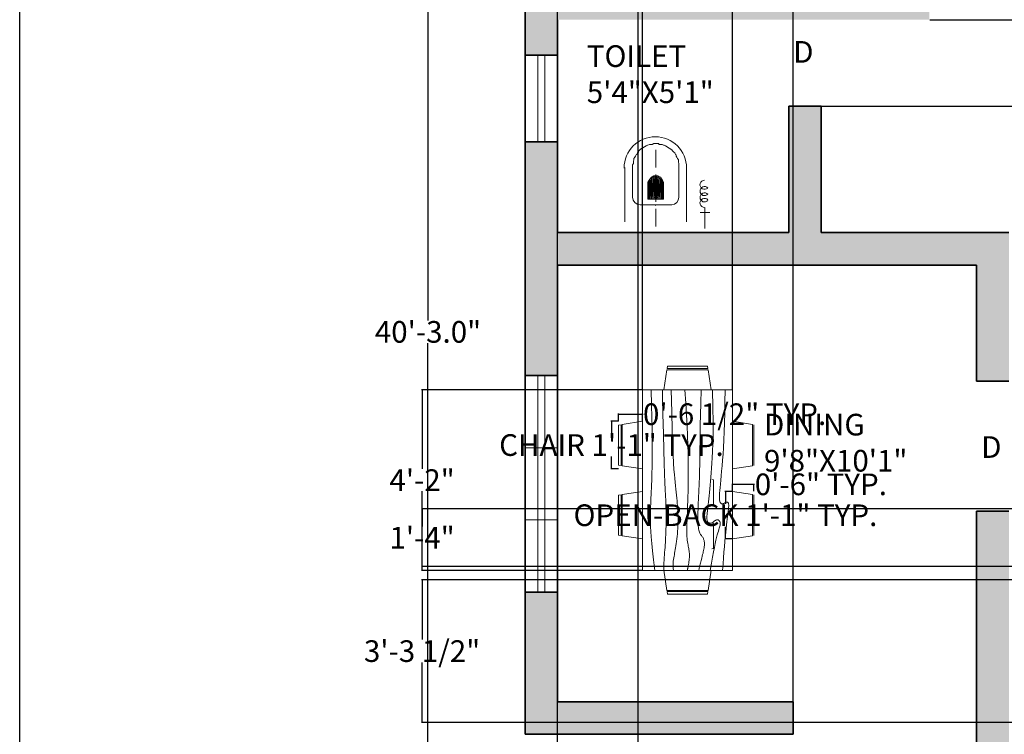
# Model space of a CAD drawing. Units: inches. Extents: x 2552 to 3196, y 4736 to 5443.
# Tile 2 of 8: x 2552 to 2824, y 4938 to 5136. Entities that reach past the tile are written whole.
import ezdxf

# ---------------------------------------------------------------- set-up
doc = ezdxf.new("R2010")
doc.units = ezdxf.units.IN
doc.header["$MEASUREMENT"] = 0
for name, color, linetype, lineweight in [('A-ANNO-DIMS', 2, 'Continuous', 18), ('A-ANNO-TTLB', 7, 'Continuous', 25), ('A-AREA-IDEN', 7, 'Continuous', 18), ('A-DOOR-IDEN', 7, 'Continuous', 18), ('A-FLOR-FIXT', 7, 'Continuous', 18), ('A-FURN', 8, 'Continuous', 18), ('A-GLAZ', 4, 'Continuous', 18), ('A-WALL', 7, 'Continuous', 35)]:
    doc.layers.add(name, color=color, linetype=linetype, lineweight=lineweight)
doc.layers.add('A-WALL-PATT', color=30, linetype='Continuous', lineweight=13, true_color=0xf8991e)
doc.styles.get("Standard").update_dxf_attribs({"font": 'arial.ttf'})
doc.dimstyles.get("Standard").update_dxf_attribs({"dimtxt": 6, "dimasz": 0.18, "dimexe": 0.18, "dimexo": 0.0625, "dimgap": 0.09, "dimtad": 0, "dimtih": 1, "dimtoh": 1, "dimdec": 1, "dimzin": 0, "dimdsep": 46, "dimlunit": 3, "dimtxsty": 'Standard', "dimcen": 0.09, "dimadec": 0, "dimazin": 0, "dimtfac": 1, "dimtdec": 1, "dimtofl": 0, "dimtmove": 0, "dimatfit": 3, "dimfxl": 1, "dimtolj": 1, "dimtzin": 0, "dimarcsym": 0})

# ---------------------------------------------------------------- blocks, each defined once
blk = doc.blocks.new('*D1')
at = {"layer": 'A-ANNO-DIMS', "color": 0, "lineweight": -2, "transparency": 16777216}
for p, q in [((2691.59, 5291.32), (2664.57, 5291.32)), ((2664.75, 5291.14), (2664.75, 5052.97)), ((2664.75, 4808.5), (2664.75, 5046.66)), ((2691.59, 4808.32), (2664.57, 4808.32))]:
    blk.add_line(p, q, dxfattribs=at)
at = {"layer": 'A-ANNO-DIMS', "color": 0, "transparency": 16777216}
for points in [[(2664.72, 5291.14), (2664.78, 5291.14), (2664.75, 5291.32)], [(2664.72, 4808.5), (2664.78, 4808.5), (2664.75, 4808.32)]]:
    blk.add_solid(points, dxfattribs=at)
at = {"layer": 'Defpoints', "color": 0, "transparency": 16777216}
for p in [(2691.66, 5291.32), (2664.75, 4808.32), (2691.66, 4808.32)]:
    blk.add_point(p, dxfattribs=at)
at = {"layer": 'A-ANNO-DIMS', "color": 0, "transparency": 16777216, "insert": (2664.75, 5049.82), "char_height": 6, "attachment_point": 5}
blk.add_mtext('\\A1;40\'-3.0"', dxfattribs=at)
blk = doc.blocks.new('WIN-60IN-THREE-LIGHT')
for p, q in [((60, 9), (0, 9)), ((20, 9), (20, 0)), ((40, 0), (40, 9)), ((60, 5.5), (0, 5.5)), ((0, 3.5), (60, 3.5)), ((0, 0), (60, 0))]:
    blk.add_line(p, q)
blk = doc.blocks.new('VENT-24IN')
for p, q in [((24, 9), (0, 9)), ((24, 5.5), (0, 5.5)), ((0, 3.5), (24, 3.5)), ((0, 0), (24, 0))]:
    blk.add_line(p, q)
blk = doc.blocks.new('WC-SQUAT')
h = blk.add_hatch(color=256)
h.paths.add_polyline_path([(7.21, 8.12), (7.21, 13.81), (7.05, 8.12)])
h.paths.add_polyline_path([(7.21, 13.81), (7.05, 8.12), (7.05, 13.58)])
h = blk.add_hatch(color=256)
h.paths.add_polyline_path([(7.59, 8.12), (7.59, 14.19), (7.21, 8.12)])
h.paths.add_polyline_path([(7.59, 14.19), (7.21, 8.12), (7.21, 13.81)])
h = blk.add_hatch(color=256)
h.paths.add_polyline_path([(7.81, 8.12), (7.81, 14.34), (7.59, 8.12)])
h.paths.add_polyline_path([(7.81, 14.34), (7.59, 8.12), (7.59, 14.19)])
h = blk.add_hatch(color=256)
h.paths.add_polyline_path([(8.19, 8.12), (8.19, 14.56), (7.81, 8.12)])
h.paths.add_polyline_path([(8.19, 14.56), (7.81, 8.12), (7.81, 14.34)])
h = blk.add_hatch(color=256)
h.paths.add_polyline_path([(8.57, 8.12), (8.57, 14.56), (8.19, 8.12)])
h.paths.add_polyline_path([(8.57, 14.56), (8.19, 8.12), (8.19, 14.56)])
h = blk.add_hatch(color=256)
h.paths.add_polyline_path([(8.95, 8.12), (8.95, 14.56), (8.57, 8.12)])
h.paths.add_polyline_path([(8.95, 14.56), (8.57, 8.12), (8.57, 14.56)])
h = blk.add_hatch(color=256)
h.paths.add_polyline_path([(9.33, 8.12), (9.33, 14.56), (8.95, 8.12)])
h.paths.add_polyline_path([(9.33, 14.56), (8.95, 8.12), (8.95, 14.56)])
h = blk.add_hatch(color=256)
h.paths.add_polyline_path([(9.71, 8.12), (9.71, 14.34), (9.33, 8.12)])
h.paths.add_polyline_path([(9.71, 14.34), (9.33, 8.12), (9.33, 14.56)])
h = blk.add_hatch(color=256)
h.paths.add_polyline_path([(10.16, 8.12), (10.16, 14.19), (9.71, 8.12)])
h.paths.add_polyline_path([(10.16, 14.19), (9.71, 8.12), (9.71, 14.34)])
h = blk.add_hatch(color=256)
h.paths.add_polyline_path([(10.32, 8.12), (10.32, 13.81), (10.16, 8.12)])
h.paths.add_polyline_path([(10.32, 13.81), (10.16, 8.12), (10.16, 14.19)])
h = blk.add_hatch(color=256)
h.paths.add_polyline_path([(10.54, 8.12), (10.54, 13.58), (10.32, 8.12)])
h.paths.add_polyline_path([(10.54, 13.58), (10.32, 8.12), (10.32, 13.81)])
h = blk.add_hatch(color=256)
h.paths.add_polyline_path([(6.83, 8.12), (6.83, 13.2), (6.6, 8.12)])
h.paths.add_polyline_path([(6.83, 13.2), (6.6, 8.12), (6.6, 12.82)])
h.paths.add_polyline_path([(6.6, 8.12), (6.6, 12.82), (6.6, 12.44)])
h = blk.add_hatch(color=256)
h.paths.add_polyline_path([(7.05, 8.12), (7.05, 13.58), (6.83, 8.12)])
h.paths.add_polyline_path([(7.05, 13.58), (6.83, 8.12), (6.83, 13.2)])
h = blk.add_hatch(color=256)
h.paths.add_polyline_path([(10.7, 8.12), (10.7, 13.2), (10.54, 8.12)])
h.paths.add_polyline_path([(10.7, 13.2), (10.54, 8.12), (10.54, 13.58)])
h = blk.add_hatch(color=256)
h.paths.add_polyline_path([(10.92, 8.12), (10.92, 12.82), (10.7, 8.12)])
h.paths.add_polyline_path([(10.92, 12.82), (10.7, 8.12), (10.7, 13.2)])
for points in [[(2.35, 15.93), (2.35, 16.69), (2.35, 17.3), (2.35, 17.67), (2.58, 18.05), (2.58, 18.43), (2.58, 18.66), (2.73, 19.04), (2.73, 19.42), (2.96, 19.8), (3.11, 20.03), (3.34, 20.41), (3.49, 20.56), (3.72, 20.94), (3.94, 21.16), (4.1, 21.54), (4.32, 21.77), (4.48, 21.92), (4.85, 22.15), (5.08, 22.3), (5.46, 22.53), (5.69, 22.68), (6.07, 22.91), (6.45, 23.14), (6.6, 23.14), (7.05, 23.29), (7.43, 23.29), (7.81, 23.29), (8.19, 23.52), (8.8, 23.52), (9.56, 23.52), (9.71, 23.29), (10.16, 23.29), (10.54, 23.29), (10.92, 23.14), (11.08, 23.14), (11.45, 22.91), (11.91, 22.68), (12.06, 22.53), (12.44, 22.3), (12.67, 22.15), (13.05, 21.92), (13.2, 21.77), (13.43, 21.54), (13.81, 21.16), (14.03, 20.94), (14.19, 20.56), (14.41, 20.41), (14.41, 20.03), (14.56, 19.8), (14.79, 19.42), (15.02, 19.04), (15.02, 18.66), (15.02, 18.43), (15.17, 18.05), (15.17, 17.67), (15.17, 17.3), (15.17, 16.69), (15.17, 15.93)], [(8.8, 16.92), (8.8, 21.77), (8.8, 21.77)], [(0.23, 1.9), (0.23, 16.92), (0.23, 16.92)], [(17.3, 1.9), (17.3, 16.92), (17.3, 16.92)], [(2.35, 8.72), (2.35, 15.93), (2.35, 15.93)], [(8.8, 7.36), (8.8, 14.94), (8.8, 14.94)], [(15.17, 8.72), (15.17, 15.93), (15.17, 15.93)], [(6.6, 8.12), (6.6, 12.44), (6.6, 12.44)], [(10.92, 8.12), (10.92, 12.44), (10.92, 12.44)], [(8.34, 8.57), (8.57, 8.57), (8.8, 8.57)], [(8.34, 8.57), (8.34, 8.5), (8.34, 8.5)], [(8.8, 8.57), (8.72, 8.5), (8.72, 8.5)], [(8.8, 8.57), (8.95, 8.57), (9.18, 8.57)], [(9.18, 8.57), (9.18, 8.5), (9.18, 8.5)], [(4.48, 6.6), (13.2, 6.6), (13.2, 6.6)], [(6.6, 8.12), (10.92, 8.12), (10.92, 8.12)], [(8.8, 6.37), (8.72, 6.37), (8.72, 6.37)], [(8.8, 0.61), (8.8, 5.46), (8.8, 5.46)], [(22.4, 0), (22.4, 5.84), (22.4, 5.84)], [(21.04, 4.48), (23.77, 4.48), (23.77, 4.48)]]:
    blk.add_lwpolyline(points)
for points in [[(7.21, 8.12), (7.21, 13.81), (7.05, 8.12)], [(7.21, 13.81), (7.05, 8.12), (7.05, 13.58)], [(7.59, 8.12), (7.59, 14.19), (7.21, 8.12)], [(7.59, 14.19), (7.21, 8.12), (7.21, 13.81)], [(7.81, 8.12), (7.81, 14.34), (7.59, 8.12)], [(7.81, 14.34), (7.59, 8.12), (7.59, 14.19)], [(8.19, 8.12), (8.19, 14.56), (7.81, 8.12)], [(8.19, 14.56), (7.81, 8.12), (7.81, 14.34)], [(8.57, 8.12), (8.57, 14.56), (8.19, 8.12)], [(8.57, 14.56), (8.19, 8.12), (8.19, 14.56)], [(8.95, 8.12), (8.95, 14.56), (8.57, 8.12)], [(8.95, 14.56), (8.57, 8.12), (8.57, 14.56)], [(9.33, 8.12), (9.33, 14.56), (8.95, 8.12)], [(9.33, 14.56), (8.95, 8.12), (8.95, 14.56)], [(9.71, 14.34), (9.33, 8.12), (9.33, 14.56)], [(9.71, 8.12), (9.71, 14.34), (9.33, 8.12)], [(10.16, 14.19), (9.71, 8.12), (9.71, 14.34)], [(10.16, 8.12), (10.16, 14.19), (9.71, 8.12)], [(10.32, 13.81), (10.16, 8.12), (10.16, 14.19)], [(10.32, 8.12), (10.32, 13.81), (10.16, 8.12)], [(10.54, 13.58), (10.32, 8.12), (10.32, 13.81)], [(6.83, 8.12), (6.83, 13.2), (6.6, 8.12)], [(6.83, 13.2), (6.6, 8.12), (6.6, 12.82)], [(6.6, 8.12), (6.6, 12.82), (6.6, 12.44)], [(6.6, 12.82), (6.6, 8.12), (6.6, 8.12)], [(7.05, 8.12), (7.05, 13.58), (6.83, 8.12)], [(7.05, 13.58), (6.83, 8.12), (6.83, 13.2)], [(10.54, 8.12), (10.54, 13.58), (10.32, 8.12)], [(10.7, 13.2), (10.54, 8.12), (10.54, 13.58)], [(10.7, 8.12), (10.7, 13.2), (10.54, 8.12)], [(10.92, 12.82), (10.7, 8.12), (10.7, 13.2)], [(10.92, 8.12), (10.92, 12.82), (10.7, 8.12)], [(10.92, 12.44), (10.92, 8.12), (10.92, 12.82)], [(10.92, 8.12), (10.92, 12.44)]]:
    blk.add_lwpolyline(points, close=True)
for points, knots in [([(17.3, 16.76), (17.3, 21.54), (13.43, 25.41), (8.65, 25.41), (8.65, 25.41), (3.87, 25.41), (0, 21.54), (0, 16.76)], [0, 0, 0, 0, 0.125, 0.125, 0.125, 0.125001, 1, 1, 1, 1]), ([(10.7, 12.29), (10.7, 13.43), (9.79, 14.34), (8.65, 14.34), (8.65, 14.34), (7.51, 14.34), (6.6, 13.43), (6.6, 12.29)], [0, 0, 0, 0, 0.125, 0.125, 0.125, 0.125001, 1, 1, 1, 1]), ([(22.25, 13.43), (21.72, 13.43), (21.19, 12.97), (21.04, 12.44), (21.04, 12.44), (20.88, 11.91), (21.19, 11.3), (21.64, 11), (21.64, 11), (22.17, 10.77), (22.78, 10.85), (23.16, 11.23)], [0, 0, 0, 0, 0.083333, 0.083333, 0.083333, 0.083334, 0.166667, 0.166667, 0.166667, 0.166668, 1, 1, 1, 1]), ([(23.23, 11.23), (22.86, 11.61), (22.32, 11.76), (21.79, 11.53), (21.79, 11.53), (21.34, 11.38), (21.04, 10.92), (21.04, 10.39), (21.04, 10.39), (21.04, 9.86), (21.34, 9.41), (21.79, 9.18), (21.79, 9.18), (22.32, 9.03), (22.86, 9.18), (23.23, 9.56)], [0, 0, 0, 0, 0.0625, 0.0625, 0.0625, 0.062501, 0.125, 0.125, 0.125, 0.125001, 0.1875, 0.1875, 0.1875, 0.187501, 1, 1, 1, 1]), ([(23.23, 7.96), (22.86, 8.34), (22.17, 8.5), (21.72, 8.19), (21.72, 8.19), (21.19, 7.89), (20.88, 7.36), (21.04, 6.75), (21.04, 6.75), (21.19, 6.22), (21.72, 5.84), (22.25, 5.84)], [0, 0, 0, 0, 0.083333, 0.083333, 0.083333, 0.083334, 0.166667, 0.166667, 0.166667, 0.166668, 1, 1, 1, 1]), ([(23.16, 9.48), (22.86, 9.86), (22.25, 10.01), (21.79, 9.79), (21.79, 9.79), (21.34, 9.63), (21.04, 9.1), (21.04, 8.65), (21.04, 8.65), (21.04, 8.12), (21.34, 7.66), (21.79, 7.43), (21.79, 7.43), (22.32, 7.28), (22.86, 7.43), (23.23, 7.81)], [0, 0, 0, 0, 0.0625, 0.0625, 0.0625, 0.062501, 0.125, 0.125, 0.125, 0.125001, 0.1875, 0.1875, 0.1875, 0.187501, 1, 1, 1, 1])]:
    blk.add_open_spline(points, degree=3, knots=knots)
for points in [[(2.35, 8.65), (2.35, 7.51), (3.26, 6.6), (4.4, 6.6)], [(13.12, 6.6), (14.26, 6.6), (15.17, 7.51), (15.17, 8.65)]]:
    blk.add_open_spline(points, degree=3)
blk = doc.blocks.new('CHAIR-DINING')
for p, q in [((0, 12.14), (0.69, 12.24)), ((0, 12.14), (0, 1.03)), ((0.69, 0.92), (0.69, 12.24)), ((1.04, 12.3), (6.6, 13.17)), ((1.04, 12.3), (1.04, 0.86)), ((0.69, 0.92), (0, 1.03)), ((6.6, 0), (1.04, 0.87))]:
    blk.add_line(p, q)
blk = doc.blocks.new('CHAIR-DINING-OPEN-BACK')
for p, q in [((5.55, 12.3), (0, 13.17)), ((5.55, 12.3), (5.55, 0.86)), ((5.9, 0.92), (5.9, 12.24)), ((0, 0), (5.55, 0.87))]:
    blk.add_line(p, q)
blk = doc.blocks.new('*D17')
at = {"layer": 'A-ANNO-DIMS', "color": 0, "lineweight": -2, "transparency": 16777216}
for p, q in [((2717.48, 5025.04), (2715.39, 5025.04)), ((2715.57, 5024.86), (2715.57, 5021.65)), ((2715.57, 5012.05), (2715.57, 5015.26)), ((2717.48, 5011.87), (2715.39, 5011.87))]:
    blk.add_line(p, q, dxfattribs=at)
at = {"layer": 'A-ANNO-DIMS', "color": 0, "transparency": 16777216}
for points in [[(2715.54, 5024.86), (2715.6, 5024.86), (2715.57, 5025.04)], [(2715.54, 5012.05), (2715.6, 5012.05), (2715.57, 5011.87)]]:
    blk.add_solid(points, dxfattribs=at)
at = {"layer": 'Defpoints', "color": 0, "transparency": 16777216}
for p in [(2715.57, 5025.04), (2717.54, 5025.04), (2717.54, 5011.87)]:
    blk.add_point(p, dxfattribs=at)
at = {"layer": 'A-ANNO-DIMS', "color": 0, "transparency": 16777216, "insert": (2715.57, 5018.46), "char_height": 6, "attachment_point": 5}
blk.add_mtext('\\A1;CHAIR 1\'-1" TYP.', dxfattribs=at)
blk = doc.blocks.new('*D18')
at = {"layer": 'A-ANNO-DIMS', "color": 0, "lineweight": -2, "transparency": 16777216}
for p, q in [((2717.54, 5025.1), (2717.54, 5027.19)), ((2717.72, 5027.01), (2723.96, 5027.01)), ((2724.14, 5025.1), (2724.14, 5027.19)), ((2724.14, 5027.01), (2724.32, 5027.01))]:
    blk.add_line(p, q, dxfattribs=at)
at = {"layer": 'A-ANNO-DIMS', "color": 0, "transparency": 16777216}
for points in [[(2717.72, 5027.04), (2717.72, 5026.98), (2717.54, 5027.01)], [(2723.96, 5027.04), (2723.96, 5026.98), (2724.14, 5027.01)]]:
    blk.add_solid(points, dxfattribs=at)
at = {"layer": 'Defpoints', "color": 0, "transparency": 16777216}
for p in [(2724.14, 5027.01), (2717.54, 5025.04), (2724.14, 5025.04)]:
    blk.add_point(p, dxfattribs=at)
at = {"layer": 'A-ANNO-DIMS', "color": 0, "transparency": 16777216, "insert": (2749.68, 5027.01), "char_height": 6, "attachment_point": 5}
blk.add_mtext('\\A1;0\'-6 1/2" TYP.', dxfattribs=at)
blk = doc.blocks.new('*D19')
at = {"layer": 'A-ANNO-DIMS', "color": 0, "lineweight": -2, "transparency": 16777216}
for p, q in [((2749.06, 5005.61), (2746.97, 5005.61)), ((2747.15, 5005.43), (2747.15, 5002.22)), ((2747.15, 4992.62), (2747.15, 4995.83)), ((2749.06, 4992.44), (2746.97, 4992.44))]:
    blk.add_line(p, q, dxfattribs=at)
at = {"layer": 'A-ANNO-DIMS', "color": 0, "transparency": 16777216}
for points in [[(2747.12, 5005.43), (2747.18, 5005.43), (2747.15, 5005.61)], [(2747.12, 4992.62), (2747.18, 4992.62), (2747.15, 4992.44)]]:
    blk.add_solid(points, dxfattribs=at)
at = {"layer": 'Defpoints', "color": 0, "transparency": 16777216}
for p in [(2747.15, 5005.61), (2749.12, 5005.61), (2749.12, 4992.44)]:
    blk.add_point(p, dxfattribs=at)
at = {"layer": 'A-ANNO-DIMS', "color": 0, "transparency": 16777216, "insert": (2747.15, 4999.02), "char_height": 6, "attachment_point": 5}
blk.add_mtext('\\A1;OPEN-BACK 1\'-1" TYP.', dxfattribs=at)
blk = doc.blocks.new('*D20')
at = {"layer": 'A-ANNO-DIMS', "color": 0, "lineweight": -2, "transparency": 16777216}
for p, q in [((2749.12, 5005.67), (2749.12, 5007.76)), ((2749.3, 5007.58), (2754.84, 5007.58)), ((2755.02, 5005.67), (2755.02, 5007.76)), ((2755.02, 5007.58), (2755.2, 5007.58))]:
    blk.add_line(p, q, dxfattribs=at)
at = {"layer": 'A-ANNO-DIMS', "color": 0, "transparency": 16777216}
for points in [[(2749.3, 5007.61), (2749.3, 5007.55), (2749.12, 5007.58)], [(2754.84, 5007.61), (2754.84, 5007.55), (2755.02, 5007.58)]]:
    blk.add_solid(points, dxfattribs=at)
at = {"layer": 'Defpoints', "color": 0, "transparency": 16777216}
for p in [(2755.02, 5007.58), (2749.12, 5005.61), (2755.02, 5005.61)]:
    blk.add_point(p, dxfattribs=at)
at = {"layer": 'A-ANNO-DIMS', "color": 0, "transparency": 16777216, "insert": (2773.58, 5007.58), "char_height": 6, "attachment_point": 5}
blk.add_mtext('\\A1;0\'-6" TYP.', dxfattribs=at)
blk = doc.blocks.new('*D26')
at = {"layer": 'A-ANNO-DIMS', "color": 0, "lineweight": -2, "transparency": 16777216}
for p, q in [((2803.72, 5136.32), (3083.39, 5136.32)), ((3083.21, 5136.14), (3083.21, 5127.47)), ((3083.21, 5112.5), (3083.21, 5121.16)), ((2773.72, 5112.32), (3083.39, 5112.32))]:
    blk.add_line(p, q, dxfattribs=at)
at = {"layer": 'A-ANNO-DIMS', "color": 0, "transparency": 16777216}
for points in [[(3083.18, 5136.14), (3083.24, 5136.14), (3083.21, 5136.32)], [(3083.18, 5112.5), (3083.24, 5112.5), (3083.21, 5112.32)]]:
    blk.add_solid(points, dxfattribs=at)
at = {"layer": 'Defpoints', "color": 0, "transparency": 16777216}
for p in [(2803.66, 5136.32), (2773.66, 5112.32), (3083.21, 5112.32)]:
    blk.add_point(p, dxfattribs=at)
at = {"layer": 'A-ANNO-DIMS', "color": 0, "transparency": 16777216, "insert": (3083.21, 5124.32), "char_height": 6, "attachment_point": 5}
blk.add_mtext('\\A1;2\'-0"', dxfattribs=at)
blk = doc.blocks.new('*D29')
at = {"layer": 'A-ANNO-DIMS', "color": 0, "lineweight": -2, "transparency": 16777216}
for p, q in [((2724.14, 5033.79), (2724.14, 5320.05)), ((2724.32, 5319.87), (2728.51, 5319.87)), ((2748.94, 5319.87), (2744.75, 5319.87)), ((2749.12, 5033.79), (2749.12, 5320.05))]:
    blk.add_line(p, q, dxfattribs=at)
at = {"layer": 'A-ANNO-DIMS', "color": 0, "transparency": 16777216}
for points in [[(2724.32, 5319.9), (2724.32, 5319.84), (2724.14, 5319.87)], [(2748.94, 5319.9), (2748.94, 5319.84), (2749.12, 5319.87)]]:
    blk.add_solid(points, dxfattribs=at)
at = {"layer": 'Defpoints', "color": 0, "transparency": 16777216}
for p in [(2749.12, 5319.87), (2724.14, 5033.73), (2749.12, 5033.73)]:
    blk.add_point(p, dxfattribs=at)
at = {"layer": 'A-ANNO-DIMS', "color": 0, "transparency": 16777216, "insert": (2736.63, 5319.87), "char_height": 6, "attachment_point": 5}
blk.add_mtext('\\A1;2\'-1"', dxfattribs=at)
blk = doc.blocks.new('*D30')
at = {"layer": 'A-ANNO-DIMS', "color": 0, "lineweight": -2, "transparency": 16777216}
for p, q in [((2724.07, 5033.73), (2662.93, 5033.73)), ((2663.11, 5033.55), (2663.11, 5011.84)), ((2663.11, 4983.93), (2663.11, 5005.64)), ((2724.07, 4983.75), (2662.93, 4983.75))]:
    blk.add_line(p, q, dxfattribs=at)
at = {"layer": 'A-ANNO-DIMS', "color": 0, "transparency": 16777216}
for points in [[(2663.08, 5033.55), (2663.14, 5033.55), (2663.11, 5033.73)], [(2663.08, 4983.93), (2663.14, 4983.93), (2663.11, 4983.75)]]:
    blk.add_solid(points, dxfattribs=at)
at = {"layer": 'Defpoints', "color": 0, "transparency": 16777216}
for p in [(2724.14, 5033.73), (2663.11, 4983.75), (2724.14, 4983.75)]:
    blk.add_point(p, dxfattribs=at)
at = {"layer": 'A-ANNO-DIMS', "color": 0, "transparency": 16777216, "insert": (2663.11, 5008.74), "char_height": 6, "attachment_point": 5}
blk.add_mtext('\\A1;4\'-2"', dxfattribs=at)
blk = doc.blocks.new('*D34')
at = {"layer": 'A-ANNO-DIMS', "color": 0, "lineweight": -2, "transparency": 16777216}
for p, q in [((2989.13, 5000.78), (2662.93, 5000.78)), ((2663.11, 5000.6), (2663.11, 4995.9)), ((2663.11, 4984.99), (2663.11, 4989.7)), ((2987.72, 4984.81), (2662.93, 4984.81))]:
    blk.add_line(p, q, dxfattribs=at)
at = {"layer": 'A-ANNO-DIMS', "color": 0, "transparency": 16777216}
for points in [[(2663.08, 5000.6), (2663.14, 5000.6), (2663.11, 5000.78)], [(2663.08, 4984.99), (2663.14, 4984.99), (2663.11, 4984.81)]]:
    blk.add_solid(points, dxfattribs=at)
at = {"layer": 'Defpoints', "color": 0, "transparency": 16777216}
for p in [(2663.11, 5000.78), (2989.19, 5000.78), (2987.78, 4984.81)]:
    blk.add_point(p, dxfattribs=at)
at = {"layer": 'A-ANNO-DIMS', "color": 0, "transparency": 16777216, "insert": (2663.11, 4992.8), "char_height": 6, "attachment_point": 5}
blk.add_mtext('\\A1;1\'-4"', dxfattribs=at)
blk = doc.blocks.new('*D35')
at = {"layer": 'A-ANNO-DIMS', "color": 0, "lineweight": -2, "transparency": 16777216}
for p, q in [((3026.66, 4981.14), (2662.93, 4981.14)), ((2663.11, 4980.96), (2663.11, 4964.56)), ((2663.11, 4941.78), (2663.11, 4958.17)), ((3026.66, 4941.6), (2662.93, 4941.6))]:
    blk.add_line(p, q, dxfattribs=at)
at = {"layer": 'A-ANNO-DIMS', "color": 0, "transparency": 16777216}
for points in [[(2663.08, 4980.96), (2663.14, 4980.96), (2663.11, 4981.14)], [(2663.08, 4941.78), (2663.14, 4941.78), (2663.11, 4941.6)]]:
    blk.add_solid(points, dxfattribs=at)
at = {"layer": 'Defpoints', "color": 0, "transparency": 16777216}
for p in [(3026.72, 4981.14), (2663.11, 4941.6), (3026.72, 4941.6)]:
    blk.add_point(p, dxfattribs=at)
at = {"layer": 'A-ANNO-DIMS', "color": 0, "transparency": 16777216, "insert": (2663.11, 4961.37), "char_height": 6, "attachment_point": 5}
blk.add_mtext('\\A1;3\'-3 1/2"', dxfattribs=at)
blk = doc.blocks.new('*D37')
at = {"layer": 'A-ANNO-DIMS', "color": 0, "lineweight": -2, "transparency": 16777216}
for p, q in [((2700.66, 4902.38), (2700.66, 5320.05)), ((2700.84, 5319.87), (2722.83, 5319.87)), ((2723.01, 4902.38), (2723.01, 5320.05)), ((2723.01, 5319.87), (2723.19, 5319.87))]:
    blk.add_line(p, q, dxfattribs=at)
at = {"layer": 'A-ANNO-DIMS', "color": 0, "transparency": 16777216}
for points in [[(2700.84, 5319.9), (2700.84, 5319.84), (2700.66, 5319.87)], [(2722.83, 5319.9), (2722.83, 5319.84), (2723.01, 5319.87)]]:
    blk.add_solid(points, dxfattribs=at)
at = {"layer": 'Defpoints', "color": 0, "transparency": 16777216}
for p in [(2723.01, 5319.87), (2700.66, 4902.32), (2723.01, 4902.32)]:
    blk.add_point(p, dxfattribs=at)
at = {"layer": 'A-ANNO-DIMS', "color": 0, "transparency": 16777216, "insert": (2740.29, 5319.87), "char_height": 6, "attachment_point": 5}
blk.add_mtext('\\A1;1\'-10 1/2"', dxfattribs=at)
blk = doc.blocks.new('*D40')
at = {"layer": 'A-ANNO-DIMS', "color": 0, "lineweight": -2, "transparency": 16777216}
for p, q in [((2700.66, 4947.38), (2700.66, 5320.05)), ((2700.84, 5319.87), (2718.23, 5319.87)), ((2765.73, 5319.87), (2748.34, 5319.87)), ((2765.91, 4947.38), (2765.91, 5320.05))]:
    blk.add_line(p, q, dxfattribs=at)
at = {"layer": 'A-ANNO-DIMS', "color": 0, "transparency": 16777216}
for points in [[(2700.84, 5319.9), (2700.84, 5319.84), (2700.66, 5319.87)], [(2765.73, 5319.9), (2765.73, 5319.84), (2765.91, 5319.87)]]:
    blk.add_solid(points, dxfattribs=at)
at = {"layer": 'Defpoints', "color": 0, "transparency": 16777216}
for p in [(2765.91, 5319.87), (2700.66, 4947.32), (2765.91, 4947.32)]:
    blk.add_point(p, dxfattribs=at)
at = {"layer": 'A-ANNO-DIMS', "color": 0, "transparency": 16777216, "insert": (2733.28, 5319.87), "char_height": 6, "attachment_point": 5}
blk.add_mtext('\\A1;5\'-5 1/2"', dxfattribs=at)

msp = doc.modelspace()

# ---------------------------------------------------------------- hatches: boundary and pattern name
at = {"layer": 'A-WALL-PATT'}
h = msp.add_hatch(color=256, dxfattribs=at)
h.dxf.hatch_style = 1
h.paths.add_polyline_path([(2700.66, 5282.32), (2732.91, 5282.32), (2732.91, 5291.32), (2691.66, 5291.32), (2691.66, 5248.4), (2700.66, 5248.4)])
h.paths.add_polyline_path([(2865.22, 5291.32), (2792.91, 5291.32), (2792.91, 5282.32), (2839.66, 5282.32), (2839.66, 5136.32), (2848.66, 5136.32), (2848.66, 5182.32), (2913.66, 5182.32), (2913.66, 5246.32), (2904.66, 5246.32), (2904.66, 5191.32), (2848.66, 5191.32), (2848.66, 5282.32), (2865.22, 5282.32)])
h.paths.add_polyline_path([(2946.08, 5291.32), (2889.22, 5291.32), (2889.22, 5282.32), (2946.08, 5282.32)])
h.paths.add_polyline_path([(3054.66, 5291.32), (3006.08, 5291.32), (3006.08, 5282.32), (3045.66, 5282.32), (3045.66, 5249.18), (3054.66, 5249.18)])
h.paths.add_polyline_path([(3054.66, 5189.18), (3045.66, 5189.18), (3045.66, 5145.32), (2904.66, 5145.32), (2904.66, 5136.32), (3045.66, 5136.32), (3045.66, 5103.54), (3054.66, 5103.54)])
h.paths.add_polyline_path([(3054.66, 5043.54), (3045.66, 5043.54), (3045.66, 5012.32), (2913.66, 5012.32), (2913.66, 5100.32), (2904.66, 5100.32), (2904.66, 5003.32), (3045.66, 5003.32), (3045.66, 4980.34), (3054.66, 4980.34)])
h.paths.add_polyline_path([(3054.66, 4920.34), (3045.66, 4920.34), (3045.66, 4886.32), (3029.6, 4886.32), (3029.6, 4877.32), (3045.66, 4877.32), (3045.66, 4817.32), (3041.59, 4817.32), (3041.59, 4808.32), (3054.66, 4808.32)])
h.paths.add_polyline_path([(2996.66, 4877.32), (3013.11, 4877.32), (3013.11, 4886.32), (2987.66, 4886.32), (2987.66, 4808.32), (2999.73, 4808.32), (2999.73, 4817.32), (2996.66, 4817.32)])
h.paths.add_polyline_path([(2825.66, 4877.32), (2853.9, 4877.32), (2853.9, 4886.32), (2825.66, 4886.32), (2825.66, 5000.12), (2816.66, 5000.12), (2816.66, 4817.32), (2785.76, 4817.32), (2785.76, 4808.32), (2825.66, 4808.32)])
h.paths.add_polyline_path([(2951.66, 4886.32), (2913.9, 4886.32), (2913.9, 4877.32), (2951.66, 4877.32)])
h.paths.add_polyline_path([(2725.76, 4817.32), (2700.66, 4817.32), (2700.66, 4833.17), (2691.66, 4833.17), (2691.66, 4808.32), (2725.76, 4808.32)])
h.paths.add_polyline_path([(2700.66, 4902.32), (2691.66, 4902.32), (2691.66, 4869.17), (2700.66, 4869.17)])
h.paths.add_polyline_path([(2765.91, 4947.32), (2700.66, 4947.32), (2700.66, 4977.71), (2691.66, 4977.71), (2691.66, 4938.32), (2765.91, 4938.32)])
h.paths.add_polyline_path([(2825.66, 5077.32), (2773.66, 5077.32), (2773.66, 5112.32), (2764.66, 5112.32), (2764.66, 5077.32), (2700.66, 5077.32), (2700.66, 5102.51), (2691.66, 5102.51), (2691.66, 5037.71), (2700.66, 5037.71), (2700.66, 5068.32), (2816.66, 5068.32), (2816.66, 5036.12), (2825.66, 5036.12)])
h.paths.add_polyline_path([(2803.66, 5145.32), (2700.66, 5145.32), (2700.66, 5188.4), (2691.66, 5188.4), (2691.66, 5126.51), (2700.66, 5126.51), (2700.66, 5136.32), (2803.66, 5136.32)])

# ---------------------------------------------------------------- linework, layer by layer
at = {"layer": 'A-ANNO-TTLB'}
msp.add_lwpolyline([(2551.65, 5442.6), (3195.75, 5442.6), (3195.75, 4736.32), (2551.65, 4736.32)], close=True, dxfattribs=at)
at = {"layer": 'A-FURN'}
for p, q in [((2730.97, 5039.63), (2731.08, 5040.32)), ((2742.18, 5040.32), (2731.08, 5040.32)), ((2742.18, 5040.32), (2742.29, 5039.63)), ((2730.05, 5033.72), (2730.91, 5039.28)), ((2742.34, 5039.28), (2730.91, 5039.28)), ((2730.97, 5039.63), (2742.29, 5039.63)), ((2742.34, 5039.28), (2743.21, 5033.72)), ((2724.14, 5033.73), (2724.14, 4983.75)), ((2749.12, 5033.73), (2724.14, 5033.73)), ((2749.12, 4983.75), (2749.12, 5033.73)), ((2743.82, 5008.85), (2743.39, 5008.92)), ((2743.82, 5008.85), (2743.82, 5001.93)), ((2743.39, 5001.86), (2743.82, 5001.93)), ((2743.82, 4996.73), (2743.39, 4996.8)), ((2743.82, 4996.73), (2743.82, 4989.81)), ((2743.39, 4989.74), (2743.82, 4989.81)), ((2724.14, 4983.75), (2749.12, 4983.75)), ((2730.05, 4983.76), (2730.91, 4978.2)), ((2742.34, 4978.2), (2743.21, 4983.76)), ((2742.34, 4978.2), (2730.91, 4978.2)), ((2730.97, 4977.85), (2742.29, 4977.85)), ((2730.97, 4977.85), (2731.08, 4977.16)), ((2742.18, 4977.16), (2742.29, 4977.85)), ((2742.18, 4977.16), (2731.08, 4977.16))]:
    msp.add_line(p, q, dxfattribs=at)
for points in [[(2726.57, 5033.73), (2726.68, 5029.62), (2726.76, 5026.11), (2726.82, 5023.13), (2726.86, 5020.59), (2726.88, 5018.44), (2726.88, 5016.58), (2726.87, 5014.97), (2726.85, 5013.51), (2726.83, 5012.16), (2726.8, 5010.88), (2726.77, 5009.69), (2726.73, 5008.57), (2726.69, 5007.52), (2726.65, 5006.52), (2726.61, 5005.58), (2726.57, 5004.69), (2726.52, 5003.84), (2726.48, 5003.02), (2726.44, 5002.22), (2726.41, 5001.42), (2726.38, 5000.61), (2726.37, 4999.77), (2726.36, 4998.89), (2726.36, 4997.95), (2726.38, 4996.95), (2726.42, 4995.82), (2726.49, 4994.53), (2726.61, 4993.01), (2726.76, 4991.23), (2726.98, 4989.12), (2727.26, 4986.65), (2727.61, 4983.75)], [(2729.69, 5033.73), (2729.82, 5027.06), (2729.95, 5021.56), (2730.07, 5017.06), (2730.19, 5013.42), (2730.3, 5010.49), (2730.4, 5008.13), (2730.48, 5006.19), (2730.56, 5004.52), (2730.61, 5003), (2730.66, 5001.59), (2730.68, 5000.29), (2730.7, 4999.1), (2730.71, 4997.99), (2730.7, 4996.97), (2730.69, 4996.02), (2730.67, 4995.15), (2730.65, 4994.33), (2730.62, 4993.56), (2730.58, 4992.83), (2730.55, 4992.13), (2730.5, 4991.45), (2730.46, 4990.78), (2730.41, 4990.11), (2730.35, 4989.42), (2730.3, 4988.72), (2730.24, 4988), (2730.19, 4987.27), (2730.14, 4986.54), (2730.1, 4985.82), (2730.06, 4985.11), (2730.04, 4984.42), (2730.04, 4983.75)], [(2732.12, 5033.73), (2732.25, 5027.61), (2732.38, 5022.68), (2732.51, 5018.78), (2732.63, 5015.76), (2732.75, 5013.44), (2732.87, 5011.68), (2732.99, 5010.31), (2733.1, 5009.17), (2733.21, 5008.14), (2733.31, 5007.16), (2733.4, 5006.25), (2733.49, 5005.39), (2733.58, 5004.57), (2733.65, 5003.79), (2733.73, 5003.04), (2733.8, 5002.32), (2733.86, 5001.61), (2733.91, 5000.92), (2733.96, 5000.23), (2734, 4999.54), (2734.02, 4998.86), (2734.04, 4998.17), (2734.04, 4997.48), (2734.03, 4996.77), (2734, 4996.04), (2733.95, 4995.31), (2733.9, 4994.58), (2733.83, 4993.85), (2733.76, 4993.14), (2733.68, 4992.45), (2733.59, 4991.78), (2733.51, 4991.16), (2733.42, 4990.57), (2733.33, 4990.02), (2733.25, 4989.5), (2733.16, 4989.01), (2733.08, 4988.54), (2733, 4988.09), (2732.92, 4987.64), (2732.84, 4987.19), (2732.77, 4986.75), (2732.7, 4986.3), (2732.65, 4985.86), (2732.62, 4985.42), (2732.62, 4984.99), (2732.64, 4984.56), (2732.71, 4984.15), (2732.81, 4983.75)], [(2735.94, 5033.73), (2736.17, 5030.11), (2736.36, 5026.8), (2736.52, 5023.77), (2736.63, 5020.99), (2736.72, 5018.46), (2736.78, 5016.13), (2736.81, 5014), (2736.83, 5012.04), (2736.84, 5010.22), (2736.83, 5008.54), (2736.81, 5006.98), (2736.78, 5005.54), (2736.75, 5004.19), (2736.71, 5002.94), (2736.67, 5001.76), (2736.63, 5000.64), (2736.59, 4999.59), (2736.55, 4998.58), (2736.51, 4997.64), (2736.48, 4996.75), (2736.45, 4995.91), (2736.44, 4995.14), (2736.44, 4994.42), (2736.46, 4993.76), (2736.49, 4993.16), (2736.53, 4992.61), (2736.58, 4992.11), (2736.64, 4991.66), (2736.71, 4991.23), (2736.78, 4990.84), (2736.85, 4990.47), (2736.92, 4990.12), (2736.98, 4989.77), (2737.04, 4989.44), (2737.08, 4989.11), (2737.12, 4988.77), (2737.15, 4988.43), (2737.16, 4988.08), (2737.16, 4987.72), (2737.15, 4987.34), (2737.12, 4986.94), (2737.08, 4986.53), (2737.03, 4986.12), (2736.97, 4985.72), (2736.91, 4985.35), (2736.85, 4985.01), (2736.79, 4984.71), (2736.74, 4984.48), (2736.71, 4984.3), (2736.68, 4984.18), (2736.66, 4984.1), (2736.64, 4984.04), (2736.64, 4983.99), (2736.63, 4983.94), (2736.63, 4983.86), (2736.63, 4983.75)], [(2740.45, 5033.73), (2740.33, 5030.06), (2740.24, 5026.83), (2740.18, 5024.01), (2740.14, 5021.53), (2740.1, 5019.36), (2740.08, 5017.45), (2740.06, 5015.76), (2740.04, 5014.23), (2740.02, 5012.84), (2739.99, 5011.56), (2739.96, 5010.37), (2739.92, 5009.25), (2739.88, 5008.2), (2739.84, 5007.2), (2739.8, 5006.23), (2739.75, 5005.27), (2739.71, 5004.32), (2739.67, 5003.37), (2739.63, 5002.44), (2739.59, 5001.54), (2739.56, 5000.67), (2739.54, 4999.84), (2739.53, 4999.05), (2739.52, 4998.33), (2739.53, 4997.67), (2739.54, 4997.07), (2739.57, 4996.52), (2739.61, 4996.04), (2739.66, 4995.6), (2739.72, 4995.21), (2739.79, 4994.87), (2739.87, 4994.57), (2739.96, 4994.31), (2740.06, 4994.07), (2740.17, 4993.87), (2740.28, 4993.69), (2740.4, 4993.52), (2740.51, 4993.37), (2740.62, 4993.22), (2740.74, 4993.07), (2740.84, 4992.91), (2740.94, 4992.75), (2741.03, 4992.58), (2741.11, 4992.39), (2741.18, 4992.2), (2741.24, 4991.98), (2741.28, 4991.75), (2741.31, 4991.5), (2741.33, 4991.23), (2741.33, 4990.94), (2741.31, 4990.63), (2741.28, 4990.31), (2741.23, 4989.97), (2741.18, 4989.63), (2741.11, 4989.27), (2741.02, 4988.9), (2740.93, 4988.53), (2740.83, 4988.12), (2740.7, 4987.66), (2740.56, 4987.13), (2740.4, 4986.5), (2740.21, 4985.74), (2740, 4984.83), (2739.75, 4983.75)], [(2743.57, 5033.73), (2743.67, 5028.85), (2743.71, 5024.82), (2743.71, 5021.53), (2743.66, 5018.85), (2743.59, 5016.68), (2743.5, 5014.9), (2743.39, 5013.4), (2743.28, 5012.07), (2743.17, 5010.8), (2743.07, 5009.59), (2742.98, 5008.43), (2742.88, 5007.33), (2742.79, 5006.29), (2742.7, 5005.31), (2742.62, 5004.39), (2742.53, 5003.53), (2742.44, 5002.74), (2742.36, 5002.01), (2742.28, 5001.35), (2742.2, 5000.74), (2742.14, 5000.18), (2742.08, 4999.69), (2742.04, 4999.24), (2742.01, 4998.85), (2741.99, 4998.5), (2742, 4998.2), (2742.01, 4997.94), (2742.04, 4997.72), (2742.09, 4997.53), (2742.15, 4997.37), (2742.22, 4997.23), (2742.3, 4997.11), (2742.39, 4997.01), (2742.49, 4996.93), (2742.6, 4996.87), (2742.72, 4996.82), (2742.84, 4996.79), (2742.96, 4996.78), (2743.09, 4996.79), (2743.22, 4996.83), (2743.35, 4996.88), (2743.48, 4996.95), (2743.61, 4997.03), (2743.74, 4997.13), (2743.87, 4997.23), (2744, 4997.33), (2744.13, 4997.43), (2744.26, 4997.52), (2744.39, 4997.6), (2744.52, 4997.67), (2744.65, 4997.72), (2744.78, 4997.76), (2744.9, 4997.78), (2745.02, 4997.77), (2745.14, 4997.74), (2745.25, 4997.69), (2745.35, 4997.61), (2745.45, 4997.51), (2745.54, 4997.38), (2745.61, 4997.24), (2745.67, 4997.07), (2745.7, 4996.89), (2745.72, 4996.69), (2745.71, 4996.48), (2745.67, 4996.25), (2745.62, 4996.01), (2745.53, 4995.73), (2745.43, 4995.42), (2745.31, 4995.05), (2745.18, 4994.63), (2745.03, 4994.13), (2744.87, 4993.56), (2744.7, 4992.89), (2744.52, 4992.11), (2744.32, 4991.19), (2744.1, 4990.12), (2743.85, 4988.86), (2743.57, 4987.4), (2743.24, 4985.7), (2742.88, 4983.75)], [(2747.04, 5033.73), (2747.02, 5030.38), (2746.98, 5027.35), (2746.91, 5024.6), (2746.82, 5022.12), (2746.72, 5019.87), (2746.6, 5017.83), (2746.48, 5015.97), (2746.35, 5014.26), (2746.22, 5012.69), (2746.09, 5011.24), (2745.97, 5009.92), (2745.85, 5008.71), (2745.75, 5007.63), (2745.66, 5006.67), (2745.59, 5005.83), (2745.54, 5005.1), (2745.5, 5004.48), (2745.49, 5003.96), (2745.5, 5003.54), (2745.52, 5003.2), (2745.56, 5002.93), (2745.62, 5002.72), (2745.69, 5002.56), (2745.77, 5002.44), (2745.86, 5002.34), (2745.96, 5002.27), (2746.07, 5002.22), (2746.18, 5002.2), (2746.29, 5002.19), (2746.41, 5002.2), (2746.52, 5002.22), (2746.64, 5002.26), (2746.74, 5002.31), (2746.84, 5002.37), (2746.94, 5002.43), (2747.03, 5002.49), (2747.12, 5002.54), (2747.21, 5002.6), (2747.3, 5002.64), (2747.39, 5002.67), (2747.47, 5002.68), (2747.56, 5002.68), (2747.64, 5002.66), (2747.72, 5002.62), (2747.79, 5002.57), (2747.86, 5002.5), (2747.92, 5002.42), (2747.97, 5002.32), (2748, 5002.2), (2748.03, 5002.06), (2748.05, 5001.9), (2748.05, 5001.71), (2748.05, 5001.49), (2748.03, 5001.23), (2748, 5000.93), (2747.97, 5000.58), (2747.92, 5000.19), (2747.86, 4999.74), (2747.79, 4999.22), (2747.71, 4998.63), (2747.63, 4997.95), (2747.53, 4997.19), (2747.43, 4996.32), (2747.33, 4995.35), (2747.22, 4994.26), (2747.1, 4993.06), (2746.98, 4991.75), (2746.86, 4990.34), (2746.73, 4988.83), (2746.61, 4987.23), (2746.48, 4985.53), (2746.35, 4983.75)]]:
    msp.add_lwpolyline(points, dxfattribs=at)
at = {"layer": 'A-WALL'}
for p, q in [((2691.66, 5291.32), (2691.66, 4938.32)), ((2700.66, 5136.32), (2700.66, 5077.32)), ((2691.66, 5126.51), (2700.66, 5126.51)), ((2764.66, 5112.32), (2773.66, 5112.32)), ((2764.66, 5112.32), (2764.66, 5077.32)), ((2773.66, 5112.32), (2773.66, 5077.32)), ((2700.66, 5102.51), (2691.66, 5102.51)), ((2700.66, 5077.32), (2764.66, 5077.32)), ((2773.66, 5077.32), (2825.66, 5077.32)), ((2700.66, 5068.32), (2816.66, 5068.32)), ((2700.66, 5068.32), (2700.66, 4947.32)), ((2816.66, 5068.32), (2816.66, 5036.12)), ((2691.66, 5037.71), (2700.66, 5037.71)), ((2816.66, 5036.12), (2825.66, 5036.12)), ((2825.66, 5000.12), (2816.66, 5000.12)), ((2816.66, 5000.12), (2816.66, 4817.32)), ((2700.66, 4977.71), (2691.66, 4977.71)), ((2700.66, 4947.32), (2765.91, 4947.32)), ((2765.91, 4947.32), (2765.91, 4938.32)), ((2691.66, 4938.32), (2765.91, 4938.32))]:
    msp.add_line(p, q, dxfattribs=at)

# ---------------------------------------------------------------- block references
at = {"layer": 'A-FLOR-FIXT'}
msp.add_blockref('WC-SQUAT', (2719.08, 5078.45), dxfattribs=at)
at = {"layer": 'A-FURN'}
for name, p in [('CHAIR-DINING', (2717.54, 5011.87)), ('CHAIR-DINING-OPEN-BACK', (2749.12, 5011.87)), ('CHAIR-DINING', (2717.54, 4992.44)), ('CHAIR-DINING-OPEN-BACK', (2749.12, 4992.44))]:
    msp.add_blockref(name, p, dxfattribs=at)
at = {"layer": 'A-GLAZ'}
for name, p, rotation in [('VENT-24IN', (2700.66, 5102.51), 90.00000000000381), ('WIN-60IN-THREE-LIGHT', (2700.66, 4977.71), 89.99999999999785)]:
    msp.add_blockref(name, p, dxfattribs=dict(at, rotation=rotation))

# ---------------------------------------------------------------- texts
at = {"layer": 'A-AREA-IDEN', "char_height": 6, "attachment_point": 1}
for s, width, insert in [('TOILET\\P5\'4"X5\'1"', 49.0662, (2708.74, 5129.22)), ('DINING\\P9\'8"X10\'1"', 55.791, (2757.83, 5027.12))]:
    msp.add_mtext_dynamic_manual_height_columns(s, width=width, gutter_width=1, heights=[0], dxfattribs=dict(at, insert=insert))
at = {"layer": 'A-DOOR-IDEN', "char_height": 6, "attachment_point": 1}
for insert in [(2765.9, 5130.4), (2817.98, 5020.91)]:
    msp.add_mtext_dynamic_manual_height_columns('D', width=10.2167, gutter_width=1, heights=[0], dxfattribs=dict(at, insert=insert))

# ---------------------------------------------------------------- dimensions: what is measured, and where the dimension line sits
at = {"layer": 'A-ANNO-DIMS'}
for base, p1, p2, picture, middle in [((2723.00559, 5319.86809), (2700.65555, 4902.31809), (2723.00559, 4902.31809), '*D37', (2740.28923, 5319.86809)), ((2765.9115, 5319.8681), (2700.6556, 4947.3181), (2765.9115, 4947.3181), '*D40', (2733.2835, 5319.8681)), ((2749.12, 5319.87), (2724.14, 5033.73), (2749.12, 5033.73), '*D29', (2736.63, 5319.87))]:
    dim = msp.add_linear_dim(base=base, p1=p1, p2=p2, dimstyle='Standard', override={"dimdec": 1, "dimlfac": 1, "dimrnd": 0, "dimzin": 1, "dimdsep": 46, "dimlunit": 4, "dimfrac": 2}, dxfattribs=at)
    dim.commit()
    dim.dimension.update_dxf_attribs({"geometry": picture, "text_midpoint": middle})
for base, p1, p2, override, picture, middle in [((2664.75, 4808.32), (2691.66, 5291.32), (2691.66, 4808.32), {"dimclrd": 0, "dimclre": 0, "dimclrt": 0}, '*D1', (2664.75, 5049.82)), ((3083.21, 5112.32), (2803.66, 5136.32), (2773.66, 5112.32), {"dimdec": 1, "dimlfac": 1, "dimrnd": 0, "dimzin": 1, "dimdsep": 46, "dimlunit": 4, "dimfrac": 2}, '*D26', (3083.21, 5124.32)), ((2663.11, 4983.75), (2724.14, 5033.73), (2724.14, 4983.75), {"dimdec": 1, "dimlfac": 1, "dimrnd": 0, "dimzin": 1, "dimdsep": 46, "dimlunit": 4, "dimfrac": 2}, '*D30', (2663.11, 5008.74)), ((2663.11, 5000.78), (2987.78, 4984.81), (2989.19, 5000.78), {"dimdec": 1, "dimlfac": 1, "dimrnd": 0, "dimzin": 1, "dimdsep": 46, "dimlunit": 4, "dimfrac": 2}, '*D34', (2663.11, 4992.8)), ((2663.11, 4941.6), (3026.72, 4981.14), (3026.72, 4941.6), {"dimdec": 1, "dimlfac": 1, "dimrnd": 0, "dimzin": 1, "dimdsep": 46, "dimlunit": 4, "dimfrac": 2}, '*D35', (2663.11, 4961.37))]:
    dim = msp.add_linear_dim(base=base, p1=p1, p2=p2, angle=90, dimstyle='Standard', override=override, dxfattribs=at)
    dim.commit()
    dim.dimension.update_dxf_attribs({"geometry": picture, "text_midpoint": middle})
for base, p1, p2, picture, middle in [((2724.14, 5027.01), (2717.54, 5025.04), (2724.14, 5025.04), '*D18', (2749.68, 5027.01)), ((2755.02, 5007.58), (2749.12, 5005.61), (2755.02, 5005.61), '*D20', (2773.58, 5007.58))]:
    dim = msp.add_linear_dim(base=base, p1=p1, p2=p2, text='<> TYP.', dimstyle='Standard', override={"dimdec": 1, "dimlfac": 1, "dimrnd": 0, "dimzin": 1, "dimdsep": 46, "dimlunit": 4, "dimfrac": 2}, dxfattribs=at)
    dim.commit()
    dim.dimension.update_dxf_attribs({"geometry": picture, "text_midpoint": middle})
for base, p1, p2, text, picture, middle in [((2715.57, 5025.04), (2717.54, 5011.87), (2717.54, 5025.04), 'CHAIR <> TYP.', '*D17', (2715.57, 5018.46)), ((2747.15, 5005.61), (2749.12, 4992.44), (2749.12, 5005.61), 'OPEN-BACK <> TYP.', '*D19', (2747.15, 4999.02))]:
    dim = msp.add_linear_dim(base=base, p1=p1, p2=p2, angle=90, text=text, dimstyle='Standard', override={"dimdec": 1, "dimlfac": 1, "dimrnd": 0, "dimzin": 1, "dimdsep": 46, "dimlunit": 4, "dimfrac": 2}, dxfattribs=at)
    dim.commit()
    dim.dimension.update_dxf_attribs({"geometry": picture, "text_midpoint": middle})

doc.saveas('drawing.dxf')
